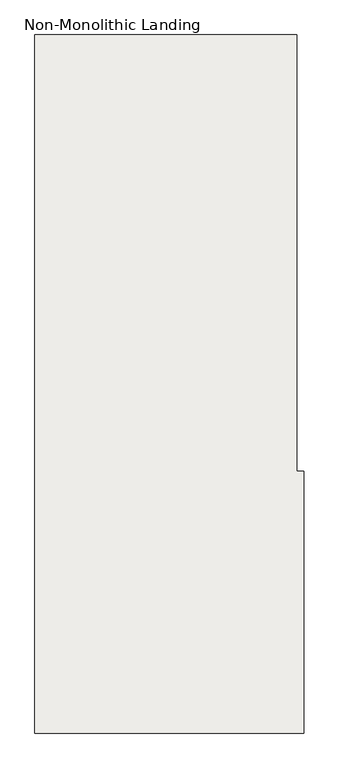
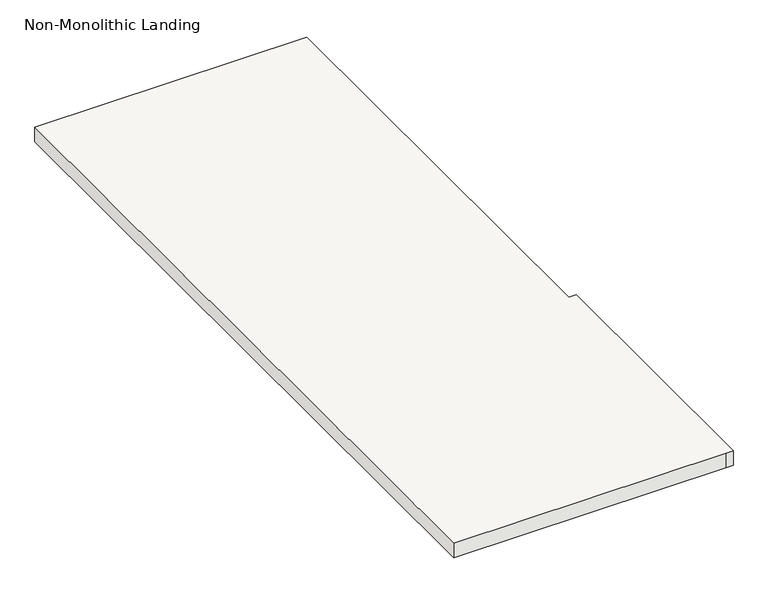
"""IFC4 building model written with IfcOpenShell, lengths in millimetres: slab geometry, Non-Monolithic Landing."""

from ifc_helpers import new_model, si_unit, origin, place, context, project, spatial, faceted_brep, source, transform, mapped, element, save


def non_monolithic_landing_c00d822c(model_context):
    return source(origin(), model_context, "Body", "Brep", [
        faceted_brep([(-8277.8763529, -1051.6338022, 8210.55), (-8252.4763529, -1051.6338022, 8235.95), (-8252.4763529, -1966.0338022, 8235.95), (-8277.8763529, -1966.0338022, 8210.55), (-9166.8763529, -1051.6338022, 8255.0), (-9166.8763529, -3490.0338022, 8255.0), (-8252.4763529, -3490.0338022, 8255.0), (-8227.0763529, -3490.0338022, 8255.0), (-8227.0763529, -2575.6338022, 8255.0), (-8252.4763529, -2575.6338022, 8255.0), (-8252.4763529, -1051.6338022, 8255.0), (-8277.8763529, -1966.0338022, 8204.2), (-8252.4763529, -1966.0338022, 8204.2), (-8252.4763529, -2575.6338022, 8204.2), (-8227.0763529, -2575.6338022, 8204.2), (-8227.0763529, -3490.0338022, 8204.2), (-8252.4763529, -3490.0338022, 8204.2), (-9166.8763529, -3490.0338022, 8204.2), (-9166.8763529, -1051.6338022, 8204.2), (-8277.8763529, -1051.6338022, 8204.2)], [[[0, 1, 2, 3]], [[4, 5, 6, 7, 8, 9, 10]], [[11, 12, 13, 14, 15, 16, 17, 18, 19]], [[12, 11, 3, 2]], [[11, 19, 0, 3]], [[4, 10, 1, 0, 19, 18]], [[5, 4, 18, 17]], [[6, 5, 17, 16]], [[7, 6, 16, 15]], [[8, 7, 15, 14]], [[9, 8, 14, 13]], [[10, 9, 13, 12, 2, 1]]]),
    ])


if __name__ == "__main__":
    model = new_model("IFC4")
    model_context = context("Model", 3, world=origin())
    ifc_project = project(units=[si_unit("LENGTHUNIT", "METRE", prefix="MILLI")], contexts=[model_context])
    site = spatial("IfcSite", under=ifc_project)
    building = spatial("IfcBuilding", under=site)
    placement = place(None, origin())
    non_monolithic_landing_shape = non_monolithic_landing_c00d822c(model_context)
    element("IfcSlab", 1, ObjectType="Non-Monolithic Landing", at=placement, inside=building, context=model_context, shape_type="MappedRepresentation", body=[
        mapped(non_monolithic_landing_shape, transform((0.0, 0.0, 0.0), x_axis=(1.0, 0.0, 0.0), y_axis=(0.0, 1.0, 0.0), z_axis=(0.0, 0.0, 1.0))),
    ])
    save(model, "model.ifc")
